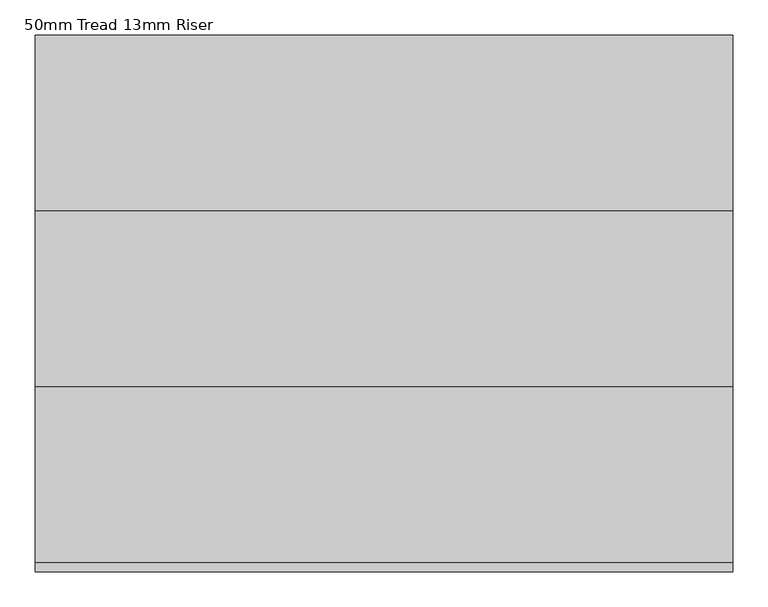
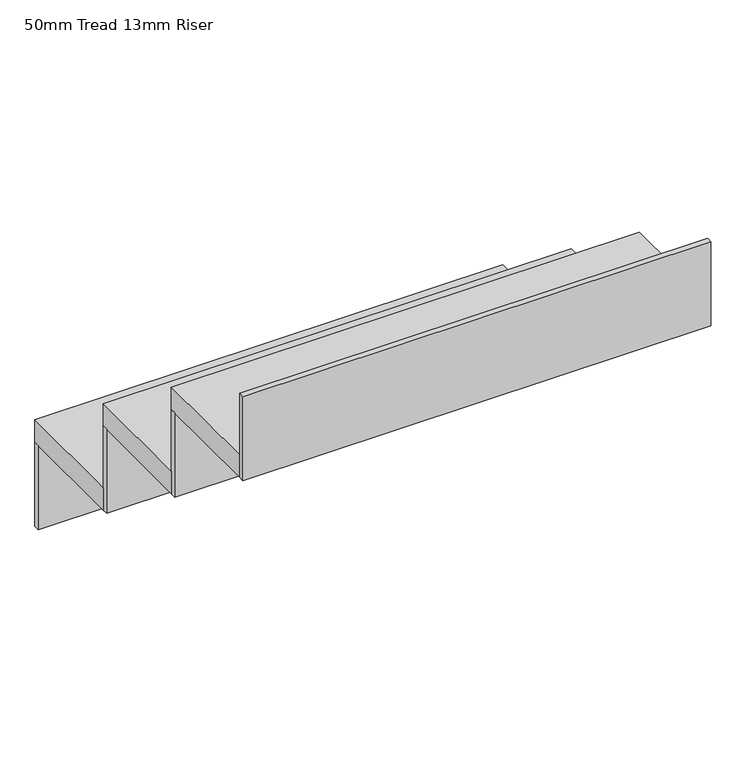
"""IFC4 building model written with IfcOpenShell, lengths in millimetres: stair flight geometry, 50mm Tread 13mm Riser."""

from ifc_helpers import new_model, si_unit, frame, origin, place, context, project, spatial, polyline, outline, extrude, source, transform, mapped, element, save


def stair_flight_50mm_tread_13mm_riser_ecc54b48(model_context):
    return source(origin(), model_context, "Body", "SweptSolid", [
        extrude(outline(polyline([(-10468.1794909, -2511.0618509), (-10468.1794909, -2498.5618509), (-9477.5794909, -2498.5618509), (-9477.5794909, -2511.0618509), (-10468.1794909, -2511.0618509)])), frame((0.0, 0.0, 1267.8117647), z_axis=(0.0, 0.0, 1.0), x_axis=(1.0, 0.0, 0.0)), (0.0, 0.0, 1.0), 188.2588235),
        extrude(outline(polyline([(-9477.5794909, -2748.5618509), (-10468.1794909, -2748.5618509), (-10468.1794909, -2498.5618509), (-9477.5794909, -2498.5618509), (-9477.5794909, -2748.5618509)])), frame((0.0, 0.0, 1456.0705882), z_axis=(0.0, 0.0, 1.0), x_axis=(1.0, 0.0, 0.0)), (0.0, 0.0, 1.0), 50.0),
        extrude(outline(polyline([(-10468.1794909, -2761.0618509), (-10468.1794909, -2748.5618509), (-9477.5794909, -2748.5618509), (-9477.5794909, -2761.0618509), (-10468.1794909, -2761.0618509)])), frame((0.0, 0.0, 1456.0705882), z_axis=(0.0, 0.0, 1.0), x_axis=(1.0, 0.0, 0.0)), (0.0, 0.0, 1.0), 188.2588235),
        extrude(outline(polyline([(-9477.5794909, -2998.5618509), (-10468.1794909, -2998.5618509), (-10468.1794909, -2748.5618509), (-9477.5794909, -2748.5618509), (-9477.5794909, -2998.5618509)])), frame((0.0, 0.0, 1644.3294118), z_axis=(0.0, 0.0, 1.0), x_axis=(1.0, 0.0, 0.0)), (0.0, 0.0, 1.0), 50.0),
        extrude(outline(polyline([(-10468.1794909, -3011.0618509), (-10468.1794909, -2998.5618509), (-9477.5794909, -2998.5618509), (-9477.5794909, -3011.0618509), (-10468.1794909, -3011.0618509)])), frame((0.0, 0.0, 1644.3294118), z_axis=(0.0, 0.0, 1.0), x_axis=(1.0, 0.0, 0.0)), (0.0, 0.0, 1.0), 188.2588235),
        extrude(outline(polyline([(-10468.1794909, -3261.0618509), (-10468.1794909, -3248.5618509), (-9477.5794909, -3248.5618509), (-9477.5794909, -3261.0618509), (-10468.1794909, -3261.0618509)])), frame((0.0, 0.0, 1832.5882353), z_axis=(0.0, 0.0, 1.0), x_axis=(1.0, 0.0, 0.0)), (0.0, 0.0, 1.0), 188.2588235),
        extrude(outline(polyline([(-9477.5794909, -3248.5618509), (-10468.1794909, -3248.5618509), (-10468.1794909, -2998.5618509), (-9477.5794909, -2998.5618509), (-9477.5794909, -3248.5618509)])), frame((0.0, 0.0, 1832.5882353), z_axis=(0.0, 0.0, 1.0), x_axis=(1.0, 0.0, 0.0)), (0.0, 0.0, 1.0), 50.0),
    ])


if __name__ == "__main__":
    model = new_model("IFC4")
    model_context = context("Model", 3, world=origin())
    ifc_project = project(units=[si_unit("LENGTHUNIT", "METRE", prefix="MILLI")], contexts=[model_context])
    site = spatial("IfcSite", under=ifc_project)
    building = spatial("IfcBuilding", under=site)
    placement = place(None, origin())
    stair_flight_50mm_tread_13mm_riser_shape = stair_flight_50mm_tread_13mm_riser_ecc54b48(model_context)
    element("IfcStairFlight", 1, ObjectType="50mm Tread 13mm Riser", at=placement, inside=building, context=model_context, shape_type="MappedRepresentation", body=[
        mapped(stair_flight_50mm_tread_13mm_riser_shape, transform((0.0, 0.0, 0.0), x_axis=(1.0, 0.0, 0.0), y_axis=(0.0, 1.0, 0.0), z_axis=(0.0, 0.0, 1.0))),
    ])
    save(model, "model.ifc")
